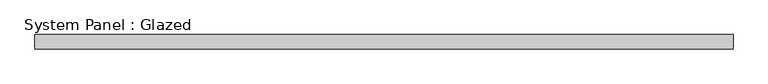
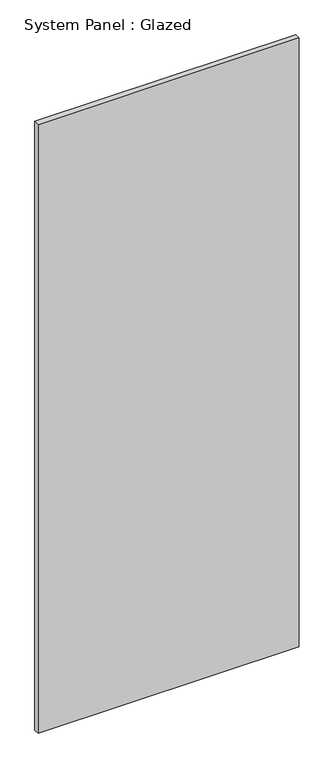
"""IFC4 building model written with IfcOpenShell, lengths in millimetres: plate geometry, System Panel : Glazed."""

from ifc_helpers import new_model, si_unit, origin, origin_with_axes, place, context, project, spatial, polyline, outline, extrude, source, transform, mapped, element, save


def system_panel_glazed_4e5522aa(model_context):
    return source(origin(), model_context, "Body", "SweptSolid", [
        extrude(outline(polyline([(609.6, 24.5), (-609.6, 24.5), (-609.6, 49.5), (609.6, 49.5), (609.6, 24.5)])), origin_with_axes(), (0.0, 0.0, 1.0), 3000.0),
    ])


if __name__ == "__main__":
    model = new_model("IFC4")
    model_context = context("Model", 3, world=origin())
    ifc_project = project(units=[si_unit("LENGTHUNIT", "METRE", prefix="MILLI")], contexts=[model_context])
    site = spatial("IfcSite", under=ifc_project)
    building = spatial("IfcBuilding", under=site)
    placement = place(None, origin())
    system_panel_glazed_shape = system_panel_glazed_4e5522aa(model_context)
    element("IfcPlate", 1, ObjectType="System Panel : Glazed", at=placement, inside=building, context=model_context, shape_type="MappedRepresentation", body=[
        mapped(system_panel_glazed_shape, transform((0.0, 0.0, 0.0), x_axis=(1.0, 0.0, 0.0), y_axis=(0.0, 1.0, 0.0), z_axis=(0.0, 0.0, 1.0))),
    ])
    save(model, "model.ifc")

# Revit data of these elements
# Type "System Panel : Glazed"
#   Keynote = "H11"
#   Construction Type Id = "GSP4R"
#   Analytic Construction = "1/8 in Pilkington single glazing"
#   Visual Light Transmittance = 0.9
#   Solar Heat Gain Coefficient = 0.86
#   Heat Transfer Coefficient (U) = 6.7069 W/(m²·K)
#   Define Thermal Properties by = 1
# Element 1 (IfcPlate, "System Panel : Glazed")
#   Materials on its faces: "Glass"
# Materials
#   "Glass": class "Glass", colour RGB 0 128 192, transparency 0.9, Description = "Soda Lime Glass", Cost = 0
